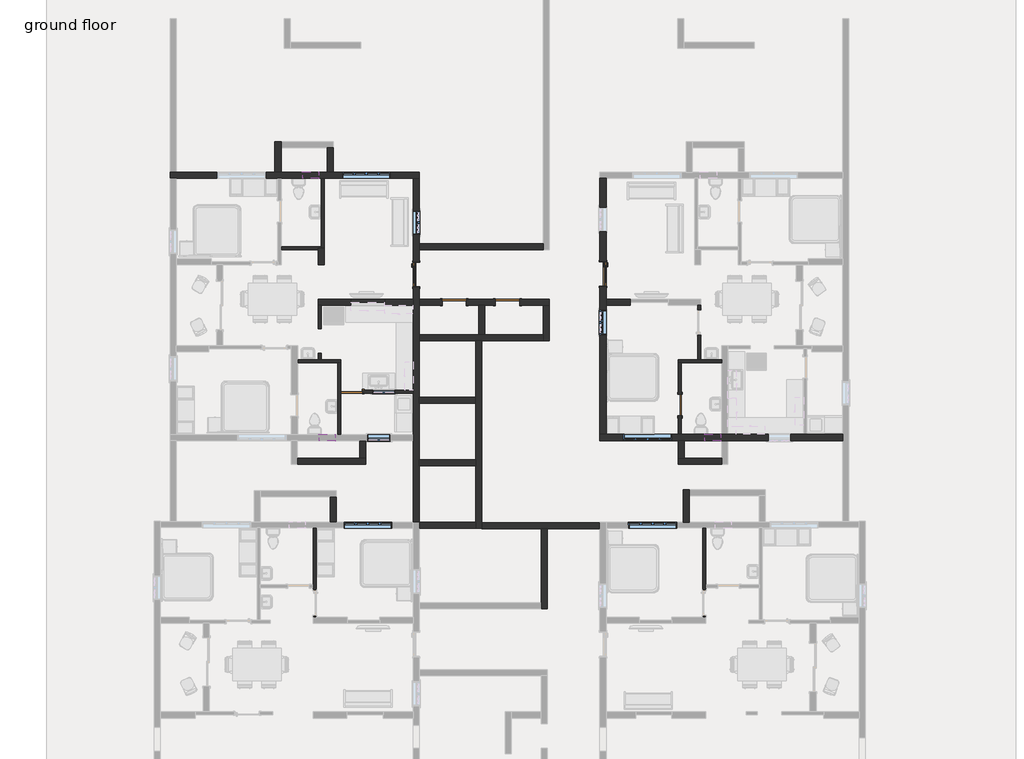
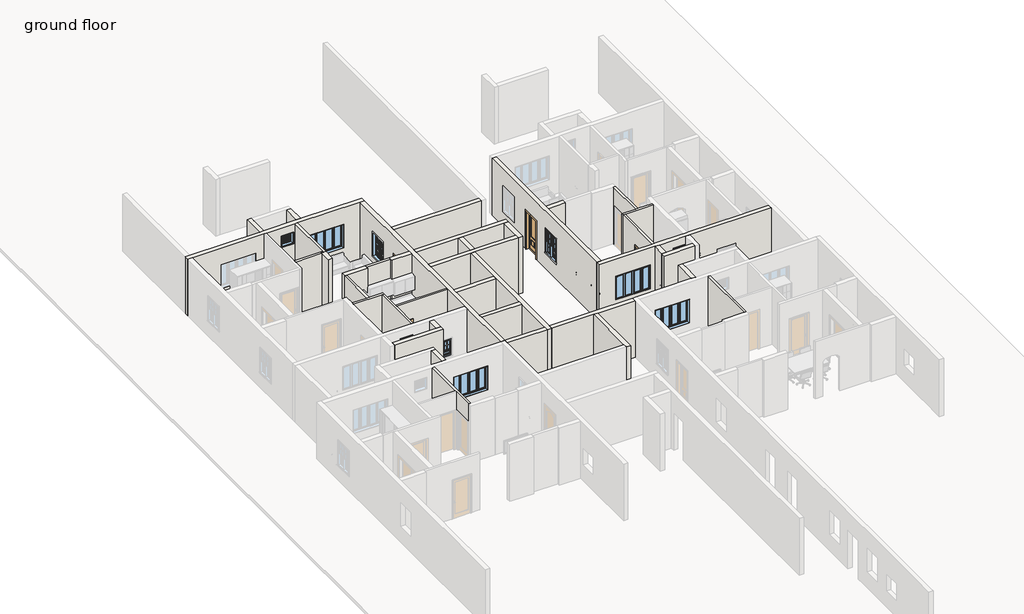
# One storey, part 5 of 16: 39 walls, 11 windows, 6 doors.
"""IFC4 building model written with IfcOpenShell, lengths in millimetres."""

from ifc_helpers import new_model, si_unit, point, frame, origin, place, context, project, spatial, polyline, ellipse_curve, trimmed, outline, extrude, faceted_brep, transform, mapped, element, save
from ifc_brep_helpers import plane_surface, extruded_surface, advanced_brep
from components import door_fe8ae985, door_f079f64e, door_38851409, door_d141acb4, door_0ca8825f, window_ced37e8f, window_622386c7, window_5487fb6d, window_f2d8fef0, window_45970670

model = new_model("IFC4")

# Units and contexts
model_context = context("Model", 3, world=origin())
ifc_project = project(units=[si_unit("LENGTHUNIT", "METRE", prefix="MILLI")], contexts=[model_context])

# Site, building, storey
site = spatial("IfcSite", under=ifc_project)
building = spatial("IfcBuilding", under=site)
storey = spatial("IfcBuildingStorey", under=building, Name="ground floor", Elevation=609.6)

# Doors
placement = place(None, origin())
door_shape = door_fe8ae985(model_context)
element("IfcDoor", 1, ObjectType="36\" x 84\"", at=placement, inside=storey, context=model_context, shape_type="MappedRepresentation", body=[
    mapped(door_shape, transform((59474.0062819, 11381.8650652, 609.6), x_axis=(0.0, 1.0, 0.0), y_axis=(-1.0, 0.0, 0.0), z_axis=(0.0, 0.0, 1.0))),
])
door_2_shape = door_f079f64e(model_context)
element("IfcDoor", 2, ObjectType="36\" x 84\"", at=placement, inside=storey, context=model_context, shape_type="MappedRepresentation", body=[
    mapped(door_2_shape, transform((52422.151243, 11359.5034272, 609.6), x_axis=(0.0, 1.0, 0.0), y_axis=(-1.0, 0.0, 0.0), z_axis=(0.0, 0.0, 1.0))),
])
door_3_shape = door_38851409(model_context)
element("IfcDoor", 3, ObjectType="Single-Flush : 32\" x 84\"", at=placement, inside=storey, context=model_context, shape_type="MappedRepresentation", body=[
    mapped(door_3_shape, transform((62372.7812819, 6428.8650652, 609.6), x_axis=(0.0, 1.0, 0.0), y_axis=(-1.0, 0.0, 0.0), z_axis=(0.0, 0.0, 1.0))),
])
door_4_shape = door_d141acb4(model_context)
element("IfcDoor", 4, ObjectType="Single-Flush : 32\" x 84\"", at=placement, inside=storey, context=model_context, shape_type="MappedRepresentation", body=[
    mapped(door_4_shape, transform((49980.576243, 6943.2150652, 609.6), x_axis=(-1.0, 0.0, 0.0), y_axis=(0.0, -1.0, 0.0), z_axis=(0.0, 0.0, 1.0))),
])
door_5_shape = door_0ca8825f(model_context)
element("IfcDoor", 5, ObjectType="Single-Flush : 36\" x 84\"", at=placement, inside=storey, context=model_context, shape_type="MappedRepresentation", body=[
    mapped(door_5_shape, transform((55864.0312819, 10315.0650652, 609.6), x_axis=(1.0, 0.0, 0.0), y_axis=(0.0, 1.0, 0.0), z_axis=(0.0, 0.0, 1.0))),
])
element("IfcDoor", 6, ObjectType="Single-Flush : 36\" x 84\"", at=placement, inside=storey, context=model_context, shape_type="MappedRepresentation", body=[
    mapped(door_5_shape, transform((53857.4312819, 10315.0650652, 609.6), x_axis=(1.0, 0.0, 0.0), y_axis=(0.0, 1.0, 0.0), z_axis=(0.0, 0.0, 1.0))),
])

# Walls
element("IfcWall", 7, ObjectType="Generic - 4.5\"", at=placement, inside=storey, context=model_context, shape_type="Brep", body=[
    faceted_brep([(48843.926243, 14998.0718163, 609.6), (48843.926243, 12410.5650652, 609.6), (48843.926243, 12353.4150652, 609.6), (48843.926243, 12353.4150652, 3810.0), (48843.926243, 12410.5650652, 3810.0), (48843.926243, 14998.0718163, 3810.0), (48958.226243, 14998.0718163, 609.6), (48958.226243, 14998.0718163, 3810.0), (48958.226243, 12353.4150652, 3810.0), (48958.226243, 12353.4150652, 609.6)], [[[0, 1, 2, 3, 4, 5]], [[6, 7, 8, 9]], [[2, 1, 0, 6, 9]], [[3, 2, 9, 8]], [[5, 4, 3, 8, 7]], [[0, 5, 7, 6]]]),
])
element("IfcWall", 8, ObjectType="Generic - 4.5\"", at=placement, inside=storey, context=model_context, shape_type="SweptSolid", body=[
    extrude(outline(polyline([(48729.626243, 12296.2650652), (47319.926243, 12296.2650652), (47319.926243, 12410.5650652), (48843.926243, 12410.5650652), (48843.926243, 12353.4150652), (48729.626243, 12353.4150652), (48729.626243, 12296.2650652)])), frame((0.0, 0.0, 609.6), z_axis=(0.0, 0.0, 1.0), x_axis=(1.0, 0.0, 0.0)), (0.0, 0.0, 1.0), 3200.4),
])
element("IfcWall", 9, ObjectType="Generic - 4.5\"", at=placement, inside=storey, context=model_context, shape_type="SweptSolid", body=[
    extrude(outline(polyline([(51230.5865418, 10315.0650652), (49954.5136957, 10315.0650652), (49954.5136957, 10429.3650652), (51230.5865418, 10429.3650652), (51230.5865418, 10315.0650652)])), frame((0.0, 0.0, 609.6), z_axis=(0.0, 0.0, 1.0), x_axis=(1.0, 0.0, 0.0)), (0.0, 0.0, 1.0), 3200.4),
])
element("IfcWall", 10, ObjectType="Generic - 4.5\"", at=placement, inside=storey, context=model_context, shape_type="AdvancedBrep", body=[
    advanced_brep(
    [(48729.626243, 10200.7650652, 609.6), (48729.626243, 9305.4150652, 609.6), (48729.626243, 9305.4150652, 2540.0), (48729.626243, 8391.0150652, 2540.0), (48729.626243, 8391.0150652, 609.6), (48729.626243, 8143.3650652, 609.6), (48729.626243, 8143.3650652, 3810.0), (48729.626243, 10200.7650652, 3810.0), (48843.926243, 9305.4150652, 2540.0), (48843.926243, 9305.4150652, 609.6), (48843.926243, 10200.7650652, 609.6), (48843.926243, 10200.7650652, 3810.0), (48843.926243, 8143.3650652, 3810.0), (48843.926243, 8143.3650652, 609.6), (48843.926243, 8391.0150652, 609.6), (48843.926243, 8391.0150652, 2540.0)],
    [
        (0, 1),
        (1, 2),
        (2, 3, ellipse_curve(frame((48729.626243, 8848.2150652, 2540.0), z_axis=(1.0, 0.0, 0.0), x_axis=(0.0, 1.0, 0.0)), 457.2, 203.2)),
        (3, 4),
        (4, 5),
        (5, 6),
        (6, 7),
        (7, 0),
        (8, 9),
        (9, 10),
        (10, 11),
        (11, 12),
        (12, 13),
        (13, 14),
        (14, 15),
        (15, 8, ellipse_curve(frame((48843.926243, 8848.2150652, 2540.0), z_axis=(-1.0, 0.0, 0.0), x_axis=(0.0, 1.0, 0.0)), 457.2, 203.2)),
        (13, 5),
        (4, 14),
        (9, 1),
        (0, 10),
        (6, 12),
        (11, 7),
        (2, 8),
        (15, 3),
    ],
    [
        plane_surface(frame((48729.626243, 10200.7650652, 609.6), z_axis=(-1.0, 0.0, 0.0), x_axis=(0.0, -1.0, 0.0))),
        plane_surface(frame((48843.926243, 10200.7650652, 609.6), z_axis=(1.0, 0.0, 0.0), x_axis=(0.0, 1.0, 0.0))),
        plane_surface(frame((48729.626243, 10315.0650652, 609.6), z_axis=(0.0, 0.0, -1.0), x_axis=(1.0, 0.0, 0.0))),
        plane_surface(frame((48729.626243, 8086.2150652, 3810.0), z_axis=(0.0, 0.0, 1.0), x_axis=(1.0, 0.0, 0.0))),
        plane_surface(frame((48729.626243, 10200.7650652, 609.6), z_axis=(0.0, 1.0, 0.0), x_axis=(1.0, 0.0, 0.0))),
        plane_surface(frame((47942.226243, 8143.3650652, 609.6), z_axis=(0.0, -1.0, 0.0), x_axis=(-1.0, 0.0, 0.0))),
        extruded_surface(trimmed(ellipse_curve(frame((48958.226243, 8848.2150652, 2540.0), z_axis=(1.0, 0.0, 0.0), x_axis=(0.0, 1.0, 0.0)), 457.2, 203.2), [point((48958.226243, 9305.4150652, 2540.0))], [point((48958.226243, 8391.0150652, 2540.0))], True, "CARTESIAN"), (-114.29999999999563, 0.0, 0.0), 114.29999999999563),
        plane_surface(frame((48729.626243, 8391.0150652, 2540.0), z_axis=(0.0, 1.0, 0.0), x_axis=(1.0, 0.0, 0.0))),
        plane_surface(frame((48729.626243, 9305.4150652, 609.6), z_axis=(0.0, -1.0, 0.0), x_axis=(1.0, 0.0, 0.0))),
    ],
    [
        (0, [[1, 2, 3, 4, 5, 6, 7, 8]]),
        (1, [[9, 10, 11, 12, 13, 14, 15, 16]]),
        (2, [[-14, 17, -5, 18]]),
        (2, [[-10, 19, -1, 20]]),
        (3, [[-7, 21, -12, 22]]),
        (4, [[-8, -22, -11, -20]]),
        (5, [[-6, -17, -13, -21]]),
        (6, [[-3, 23, -16, 24]]),
        (7, [[-4, -24, -15, -18]]),
        (8, [[-2, -19, -9, -23]]),
    ],
),
])
element("IfcWall", 11, ObjectType="Generic - 4.5\"", at=placement, inside=storey, context=model_context, shape_type="Brep", body=[
    faceted_brep([(47942.226243, 8029.0650652, 609.6), (49466.226243, 8029.0650652, 609.6), (49580.526243, 8029.0650652, 609.6), (49580.526243, 8029.0650652, 3810.0), (49466.226243, 8029.0650652, 3810.0), (47942.226243, 8029.0650652, 3810.0), (47942.226243, 8143.3650652, 609.6), (47942.226243, 8143.3650652, 3810.0), (48729.626243, 8143.3650652, 3810.0), (48843.926243, 8143.3650652, 3810.0), (49580.526243, 8143.3650652, 3810.0), (49580.526243, 8143.3650652, 609.6), (48843.926243, 8143.3650652, 609.6), (48729.626243, 8143.3650652, 609.6)], [[[0, 1, 2, 3, 4, 5]], [[6, 7, 8, 9, 10, 11, 12, 13]], [[2, 1, 0, 6, 13, 12, 11]], [[5, 4, 3, 10, 9, 8, 7]], [[0, 5, 7, 6]], [[3, 2, 11, 10]]]),
])
element("IfcWall", 12, ObjectType="Generic - 4.5\"", at=placement, inside=storey, context=model_context, shape_type="Brep", body=[
    faceted_brep([(49466.226243, 8029.0650652, 609.6), (49466.226243, 5320.6718163, 609.6), (49466.226243, 5320.6718163, 3810.0), (49466.226243, 8029.0650652, 3810.0), (49580.526243, 8029.0650652, 3810.0), (49580.526243, 7000.3650652, 3810.0), (49580.526243, 6886.0650652, 3810.0), (49580.526243, 5320.6718163, 3810.0), (49580.526243, 5320.6718163, 609.6), (49580.526243, 6886.0650652, 609.6), (49580.526243, 6886.0650652, 2743.2), (49580.526243, 7000.3650652, 2743.2), (49580.526243, 7000.3650652, 609.6), (49580.526243, 8029.0650652, 609.6), (49574.176243, 7000.3650652, 609.6), (49574.176243, 6886.0650652, 609.6), (49574.176243, 7000.3650652, 2743.2), (49574.176243, 6886.0650652, 2743.2)], [[[0, 1, 2, 3]], [[4, 5, 6, 7, 8, 9, 10, 11, 12, 13]], [[1, 0, 13, 12, 14, 15, 9, 8]], [[3, 2, 7, 6, 5, 4]], [[0, 3, 4, 13]], [[2, 1, 8, 7]], [[16, 14, 12, 11]], [[15, 17, 10, 9]], [[14, 16, 17, 15]], [[17, 16, 11, 10]]]),
])
element("IfcWall", 13, ObjectType="Generic - 4.5\"", at=placement, inside=storey, context=model_context, shape_type="SweptSolid", body=[
    extrude(outline(polyline([(3810.0, 52311.026243), (3810.0, 49580.526243), (2743.2, 49580.526243), (2743.2, 50386.976243), (609.6, 50386.976243), (609.6, 52311.026243), (3810.0, 52311.026243)]), holes=[polyline([(2438.4, 50771.151243), (2438.4, 51634.751243), (1524.0, 51634.751243), (1524.0, 50771.151243), (2438.4, 50771.151243)])]), frame((0.0, 6886.0650652, 0.0), z_axis=(0.0, 1.0, 0.0), x_axis=(0.0, 0.0, 1.0)), (0.0, 0.0, 1.0), 114.3),
])
element("IfcWall", 14, ObjectType="Generic - 4.5\"", at=placement, inside=storey, context=model_context, shape_type="Brep", body=[
    faceted_brep([(63953.9312819, 8143.3650652, 609.6), (63166.5312819, 8143.3650652, 609.6), (63052.2312819, 8143.3650652, 609.6), (62315.6312819, 8143.3650652, 609.6), (62315.6312819, 8143.3650652, 3810.0), (63052.2312819, 8143.3650652, 3810.0), (63166.5312819, 8143.3650652, 3810.0), (63953.9312819, 8143.3650652, 3810.0), (63953.9312819, 8029.0650652, 609.6), (63953.9312819, 8029.0650652, 3810.0), (62429.9312819, 8029.0650652, 3810.0), (62315.6312819, 8029.0650652, 3810.0), (62315.6312819, 8029.0650652, 609.6), (62429.9312819, 8029.0650652, 609.6)], [[[0, 1, 2, 3, 4, 5, 6, 7]], [[8, 9, 10, 11, 12, 13]], [[3, 2, 1, 0, 8, 13, 12]], [[7, 6, 5, 4, 11, 10, 9]], [[0, 7, 9, 8]], [[4, 3, 12, 11]]]),
])
element("IfcWall", 15, ObjectType="Generic - 4.5\"", at=placement, inside=storey, context=model_context, shape_type="SweptSolid", body=[
    extrude(outline(polyline([(8029.0650652, 609.6), (6835.2650652, 609.6), (6835.2650652, 2743.2), (6022.4650652, 2743.2), (6022.4650652, 609.6), (5323.9650652, 609.6), (5323.9650652, 3810.0), (8029.0650652, 3810.0), (8029.0650652, 609.6)])), frame((62315.6312819, 0.0, 0.0), z_axis=(1.0, 0.0, 0.0), x_axis=(0.0, 1.0, 0.0)), (0.0, 0.0, 1.0), 114.3),
])
element("IfcWall", 16, ObjectType="Generic - 4.5\"", at=placement, inside=storey, context=model_context, shape_type="SweptSolid", body=[
    extrude(outline(polyline([(8143.3650652, 3810.0), (10200.7650652, 3810.0), (10200.7650652, 609.6), (10035.6650652, 609.6), (10035.6650652, 2768.6), (9070.4650652, 2768.6), (9070.4650652, 609.6), (8143.3650652, 609.6), (8143.3650652, 3810.0)])), frame((63052.2312819, 0.0, 0.0), z_axis=(1.0, 0.0, 0.0), x_axis=(0.0, 1.0, 0.0)), (0.0, 0.0, 1.0), 114.3),
])
element("IfcWall", 17, ObjectType="Generic - 4.5\"", at=placement, inside=storey, context=model_context, shape_type="Brep", body=[
    faceted_brep([(48539.126243, -1566.0113664, 3810.0), (48539.126243, -461.1113664, 3810.0), (48539.126243, -346.8113664, 3810.0), (48539.126243, 1794.3724636, 3810.0), (48539.126243, 1794.3724636, 609.6), (48539.126243, -346.8113664, 609.6), (48539.126243, -461.1113664, 609.6), (48539.126243, -559.5363664, 609.6), (48539.126243, -559.5363664, 2768.6), (48539.126243, -1524.7363664, 2768.6), (48539.126243, -1524.7363664, 609.6), (48539.126243, -1566.0113664, 609.6), (48653.426243, 1793.9176995, 3810.0), (48653.426243, -1566.0113664, 3810.0), (48653.426243, -1566.0113664, 609.6), (48653.426243, -1524.7363664, 609.6), (48653.426243, -1524.7363664, 2768.6), (48653.426243, -559.5363664, 2768.6), (48653.426243, -559.5363664, 609.6), (48653.426243, 1793.9176995, 609.6)], [[[0, 1, 2, 3, 4, 5, 6, 7, 8, 9, 10, 11]], [[12, 13, 14, 15, 16, 17, 18, 19]], [[4, 19, 18, 7, 6, 5]], [[14, 11, 10, 15]], [[3, 2, 1, 0, 13, 12]], [[0, 11, 14, 13]], [[4, 3, 12, 19]], [[9, 16, 15, 10]], [[16, 9, 8, 17]], [[17, 8, 7, 18]]]),
])
element("IfcWall", 18, ObjectType="Generic - 4.5\"", at=placement, inside=storey, context=model_context, shape_type="Brep", body=[
    faceted_brep([(63242.7312819, -1566.0113664, 3810.0), (63242.7312819, 1793.9176995, 3810.0), (63242.7312819, 1793.9176995, 609.6), (63242.7312819, -559.5363664, 609.6), (63242.7312819, -559.5363664, 2768.6), (63242.7312819, -1524.7363664, 2768.6), (63242.7312819, -1524.7363664, 609.6), (63242.7312819, -1566.0113664, 609.6), (63357.0312819, 1794.3724636, 3810.0), (63357.0312819, -346.8113664, 3810.0), (63357.0312819, -461.1113664, 3810.0), (63357.0312819, -1566.0113664, 3810.0), (63357.0312819, -1566.0113664, 609.6), (63357.0312819, -1524.7363664, 609.6), (63357.0312819, -1524.7363664, 2768.6), (63357.0312819, -559.5363664, 2768.6), (63357.0312819, -559.5363664, 609.6), (63357.0312819, -461.1113664, 609.6), (63357.0312819, -346.8113664, 609.6), (63357.0312819, 1794.3724636, 609.6)], [[[0, 1, 2, 3, 4, 5, 6, 7]], [[8, 9, 10, 11, 12, 13, 14, 15, 16, 17, 18, 19]], [[2, 19, 18, 17, 16, 3]], [[12, 7, 6, 13]], [[1, 0, 11, 10, 9, 8]], [[0, 7, 12, 11]], [[2, 1, 8, 19]], [[5, 14, 13, 6]], [[14, 5, 4, 15]], [[15, 4, 3, 16]]]),
])
element("IfcWall", 19, ObjectType="Generic - 9\"", at=placement, inside=storey, context=model_context, shape_type="Brep", body=[
    faceted_brep([(43141.626243, 14998.0718163, 609.6), (43370.226243, 14998.0718163, 609.6), (47205.626243, 14998.0718163, 609.6), (47319.926243, 14998.0718163, 609.6), (48843.926243, 14998.0718163, 609.6), (48958.226243, 14998.0718163, 609.6), (52311.026243, 14998.0718163, 609.6), (52539.626243, 14998.0718163, 609.6), (52539.626243, 14998.0718163, 3810.0), (52311.026243, 14998.0718163, 3810.0), (48958.226243, 14998.0718163, 3810.0), (48843.926243, 14998.0718163, 3810.0), (47319.926243, 14998.0718163, 3810.0), (47205.626243, 14998.0718163, 3810.0), (43370.226243, 14998.0718163, 3810.0), (43141.626243, 14998.0718163, 3810.0), (46748.426243, 14998.0718163, 2870.2), (46748.426243, 14998.0718163, 1524.0), (44919.626243, 14998.0718163, 1524.0), (44919.626243, 14998.0718163, 2870.2), (51457.2877548, 14998.0718163, 2870.2), (51457.2877548, 14998.0718163, 1524.0), (49628.4877548, 14998.0718163, 1524.0), (49628.4877548, 14998.0718163, 2870.2), (48139.076243, 14998.0718163, 3352.8), (48748.676243, 14998.0718163, 3352.8), (48748.676243, 14998.0718163, 2743.2), (48139.076243, 14998.0718163, 2743.2), (43141.626243, 15226.6718163, 609.6), (43141.626243, 15226.6718163, 3810.0), (43370.226243, 15226.6718163, 3810.0), (47091.326243, 15226.6718163, 3810.0), (47319.926243, 15226.6718163, 3810.0), (49056.9877548, 15226.6718163, 3810.0), (49285.5877548, 15226.6718163, 3810.0), (52539.626243, 15226.6718163, 3810.0), (52539.626243, 15226.6718163, 609.6), (49285.5877548, 15226.6718163, 609.6), (49056.9877548, 15226.6718163, 609.6), (47319.926243, 15226.6718163, 609.6), (47091.326243, 15226.6718163, 609.6), (43370.226243, 15226.6718163, 609.6), (46748.426243, 15226.6718163, 2870.2), (44919.626243, 15226.6718163, 2870.2), (44919.626243, 15226.6718163, 1524.0), (46748.426243, 15226.6718163, 1524.0), (51457.2877548, 15226.6718163, 2870.2), (49628.4877548, 15226.6718163, 2870.2), (49628.4877548, 15226.6718163, 1524.0), (51457.2877548, 15226.6718163, 1524.0), (48139.076243, 15226.6718163, 3352.8), (48139.076243, 15226.6718163, 2743.2), (48748.676243, 15226.6718163, 2743.2), (48748.676243, 15226.6718163, 3352.8)], [[[0, 1, 2, 3, 4, 5, 6, 7, 8, 9, 10, 11, 12, 13, 14, 15], [16, 17, 18, 19], [20, 21, 22, 23], [24, 25, 26, 27]], [[28, 29, 30, 31, 32, 33, 34, 35, 36, 37, 38, 39, 40, 41], [42, 43, 44, 45], [46, 47, 48, 49], [50, 51, 52, 53]], [[7, 6, 5, 4, 3, 2, 1, 0, 28, 41, 40, 39, 38, 37, 36]], [[15, 14, 13, 12, 11, 10, 9, 8, 35, 34, 33, 32, 31, 30, 29]], [[8, 7, 36, 35]], [[0, 15, 29, 28]], [[17, 16, 42, 45]], [[18, 17, 45, 44]], [[19, 18, 44, 43]], [[16, 19, 43, 42]], [[21, 20, 46, 49]], [[22, 21, 49, 48]], [[23, 22, 48, 47]], [[20, 23, 47, 46]], [[51, 50, 24, 27]], [[52, 51, 27, 26]], [[53, 52, 26, 25]], [[50, 53, 25, 24]]]),
])
element("IfcWall", 20, ObjectType="Generic - 9\"", at=placement, inside=storey, context=model_context, shape_type="Brep", body=[
    faceted_brep([(52311.026243, 2007.967056, 3810.0), (52311.026243, 5092.0718163, 3810.0), (52311.026243, 5320.6718163, 3810.0), (52311.026243, 6886.0650652, 3810.0), (52311.026243, 7000.3650652, 3810.0), (52311.026243, 10200.7650652, 3810.0), (52311.026243, 10429.3650652, 3810.0), (52311.026243, 14998.0718163, 3810.0), (52311.026243, 14998.0718163, 609.6), (52311.026243, 11842.1034272, 609.6), (52311.026243, 11842.1034272, 2768.6), (52311.026243, 10876.9034272, 2768.6), (52311.026243, 10876.9034272, 609.6), (52311.026243, 10429.3650652, 609.6), (52311.026243, 10200.7650652, 609.6), (52311.026243, 7000.3650652, 609.6), (52311.026243, 6886.0650652, 609.6), (52311.026243, 5320.6718163, 609.6), (52311.026243, 5092.0718163, 609.6), (52311.026243, 2007.967056, 609.6), (52311.026243, 13775.5417893, 2844.8), (52311.026243, 12861.1417893, 2844.8), (52311.026243, 12861.1417893, 1524.0), (52311.026243, 13775.5417893, 1524.0), (52539.626243, 14998.0718163, 3810.0), (52539.626243, 12518.2417893, 3810.0), (52539.626243, 12289.6417893, 3810.0), (52539.626243, 10429.3650652, 3810.0), (52539.626243, 10200.7650652, 3810.0), (52539.626243, 9093.6575277, 3810.0), (52539.626243, 8865.0575277, 3810.0), (52539.626243, 6731.4575277, 3810.0), (52539.626243, 6502.8575277, 3810.0), (52539.626243, 4369.2575277, 3810.0), (52539.626243, 4140.6575277, 3810.0), (52539.626243, 2007.0575277, 3810.0), (52539.626243, 2007.0575277, 609.6), (52539.626243, 4140.6575277, 609.6), (52539.626243, 4369.2575277, 609.6), (52539.626243, 6502.8575277, 609.6), (52539.626243, 6731.4575277, 609.6), (52539.626243, 8865.0575277, 609.6), (52539.626243, 9093.6575277, 609.6), (52539.626243, 10200.7650652, 609.6), (52539.626243, 10429.3650652, 609.6), (52539.626243, 10876.9034272, 609.6), (52539.626243, 10876.9034272, 2768.6), (52539.626243, 11842.1034272, 2768.6), (52539.626243, 11842.1034272, 609.6), (52539.626243, 12289.6417893, 609.6), (52539.626243, 12518.2417893, 609.6), (52539.626243, 14998.0718163, 609.6), (52539.626243, 13775.5417893, 2844.8), (52539.626243, 13775.5417893, 1524.0), (52539.626243, 12861.1417893, 1524.0), (52539.626243, 12861.1417893, 2844.8)], [[[0, 1, 2, 3, 4, 5, 6, 7, 8, 9, 10, 11, 12, 13, 14, 15, 16, 17, 18, 19], [20, 21, 22, 23]], [[24, 25, 26, 27, 28, 29, 30, 31, 32, 33, 34, 35, 36, 37, 38, 39, 40, 41, 42, 43, 44, 45, 46, 47, 48, 49, 50, 51], [52, 53, 54, 55]], [[8, 51, 50, 49, 48, 9]], [[36, 19, 18, 17, 16, 15, 14, 13, 12, 45, 44, 43, 42, 41, 40, 39, 38, 37]], [[7, 6, 5, 4, 3, 2, 1, 0, 35, 34, 33, 32, 31, 30, 29, 28, 27, 26, 25, 24]], [[8, 7, 24, 51]], [[0, 19, 36, 35]], [[47, 10, 9, 48]], [[10, 47, 46, 11]], [[11, 46, 45, 12]], [[53, 52, 20, 23]], [[54, 53, 23, 22]], [[55, 54, 22, 21]], [[52, 55, 21, 20]]]),
])
element("IfcWall", 21, ObjectType="Generic - 9\"", at=placement, inside=storey, context=model_context, shape_type="Brep", body=[
    faceted_brep([(48729.626243, 10200.7650652, 609.6), (48843.926243, 10200.7650652, 609.6), (49954.5136957, 10200.7650652, 609.6), (49954.5136957, 10200.7650652, 3810.0), (48843.926243, 10200.7650652, 3810.0), (48729.626243, 10200.7650652, 3810.0), (48729.626243, 10429.3650652, 609.6), (48729.626243, 10429.3650652, 3810.0), (49954.5136957, 10429.3650652, 3810.0), (49954.5136957, 10429.3650652, 609.6), (49954.5136957, 10315.0650652, 609.6), (49954.5136957, 10315.0650652, 3810.0)], [[[0, 1, 2, 3, 4, 5]], [[6, 7, 8, 9]], [[2, 1, 0, 6, 9, 10]], [[3, 2, 10, 9, 8, 11]], [[5, 4, 3, 11, 8, 7]], [[0, 5, 7, 6]]]),
])
element("IfcWall", 22, ObjectType="Generic - 9\"", at=placement, inside=storey, context=model_context, shape_type="Brep", body=[
    faceted_brep([(51230.5865418, 10200.7650652, 609.6), (52311.026243, 10200.7650652, 609.6), (52311.026243, 10200.7650652, 3810.0), (51230.5865418, 10200.7650652, 3810.0), (51230.5865418, 10429.3650652, 609.6), (51230.5865418, 10429.3650652, 3810.0), (52311.026243, 10429.3650652, 3810.0), (52311.026243, 10429.3650652, 609.6), (51230.5865418, 10315.0650652, 609.6), (51230.5865418, 10315.0650652, 3810.0)], [[[0, 1, 2, 3]], [[4, 5, 6, 7]], [[1, 0, 8, 4, 7]], [[3, 2, 6, 5, 9]], [[0, 3, 9, 5, 4, 8]], [[2, 1, 7, 6]]]),
])
element("IfcWall", 23, ObjectType="Generic - 9\"", at=placement, inside=storey, context=model_context, shape_type="Brep", body=[
    faceted_brep([(48958.226243, 11724.7650652, 609.6), (48958.226243, 12353.4150652, 609.6), (48958.226243, 12353.4150652, 3810.0), (48958.226243, 11724.7650652, 3810.0), (48729.626243, 11724.7650652, 609.6), (48729.626243, 11724.7650652, 3810.0), (48729.626243, 12296.2650652, 3810.0), (48729.626243, 12353.4150652, 3810.0), (48729.626243, 12353.4150652, 609.6), (48729.626243, 12296.2650652, 609.6), (48843.926243, 12353.4150652, 609.6), (48843.926243, 12353.4150652, 3810.0)], [[[0, 1, 2, 3]], [[4, 5, 6, 7, 8, 9]], [[1, 0, 4, 9, 8, 10]], [[2, 1, 10, 8, 7, 11]], [[3, 2, 11, 7, 6, 5]], [[0, 3, 5, 4]]]),
])
element("IfcWall", 24, ObjectType="Generic - 9\"", at=placement, inside=storey, context=model_context, shape_type="Brep", body=[
    faceted_brep([(47319.926243, 15226.6718163, 609.6), (47319.926243, 16147.8755101, 609.6), (47319.926243, 16376.4755101, 609.6), (47319.926243, 16376.4755101, 3810.0), (47319.926243, 16147.8755101, 3810.0), (47319.926243, 15226.6718163, 3810.0), (47091.326243, 15226.6718163, 609.6), (47091.326243, 15226.6718163, 3810.0), (47091.326243, 16376.4755101, 3810.0), (47091.326243, 16376.4755101, 609.6)], [[[0, 1, 2, 3, 4, 5]], [[6, 7, 8, 9]], [[2, 1, 0, 6, 9]], [[5, 4, 3, 8, 7]], [[0, 5, 7, 6]], [[3, 2, 9, 8]]]),
])
element("IfcWall", 25, ObjectType="Generic - 9\"", at=placement, inside=storey, context=model_context, shape_type="SweptSolid", body=[
    extrude(outline(polyline([(49056.9877548, 15226.6718163), (49056.9877548, 16147.8755101), (49285.5877548, 16147.8755101), (49285.5877548, 15226.6718163), (49056.9877548, 15226.6718163)])), frame((0.0, 0.0, 609.6), z_axis=(0.0, 0.0, 1.0), x_axis=(1.0, 0.0, 0.0)), (0.0, 0.0, 1.0), 3200.4),
])
element("IfcWall", 26, ObjectType="Generic - 9\"", at=placement, inside=storey, context=model_context, shape_type="Brep", body=[
    faceted_brep([(47929.526243, 4203.0718163, 609.6), (50519.795833, 4203.0718163, 609.6), (50519.795833, 4203.0718163, 3810.0), (47929.526243, 4203.0718163, 3810.0), (47929.526243, 4431.6718163, 609.6), (47929.526243, 4431.6718163, 3810.0), (50291.195833, 4431.6718163, 3810.0), (50519.795833, 4431.6718163, 3810.0), (50519.795833, 4431.6718163, 609.6), (50291.195833, 4431.6718163, 609.6)], [[[0, 1, 2, 3]], [[4, 5, 6, 7, 8, 9]], [[1, 0, 4, 9, 8]], [[3, 2, 7, 6, 5]], [[0, 3, 5, 4]], [[2, 1, 8, 7]]]),
])
element("IfcWall", 27, ObjectType="Generic - 9\"", at=placement, inside=storey, context=model_context, shape_type="SweptSolid", body=[
    extrude(outline(polyline([(50519.795833, 5092.0718163), (50519.795833, 4431.6718163), (50291.195833, 4431.6718163), (50291.195833, 5092.0718163), (50519.795833, 5092.0718163)])), frame((0.0, 0.0, 609.6), z_axis=(0.0, 0.0, 1.0), x_axis=(1.0, 0.0, 0.0)), (0.0, 0.0, 1.0), 3200.4),
])
element("IfcWall", 28, ObjectType="Generic - 9\"", at=placement, inside=storey, context=model_context, shape_type="Brep", body=[
    faceted_brep([(68525.9312819, 5323.9650652, 609.6), (67154.3312819, 5323.9650652, 609.6), (67040.0312819, 5323.9650652, 609.6), (64182.5312819, 5323.9650652, 609.6), (63953.9312819, 5323.9650652, 609.6), (62429.9312819, 5323.9650652, 609.6), (62315.6312819, 5323.9650652, 609.6), (59585.1312819, 5323.9650652, 609.6), (59356.5312819, 5323.9650652, 609.6), (59356.5312819, 5323.9650652, 3810.0), (59585.1312819, 5323.9650652, 3810.0), (62315.6312819, 5323.9650652, 3810.0), (62429.9312819, 5323.9650652, 3810.0), (63953.9312819, 5323.9650652, 3810.0), (64182.5312819, 5323.9650652, 3810.0), (67040.0312819, 5323.9650652, 3810.0), (67154.3312819, 5323.9650652, 3810.0), (68525.9312819, 5323.9650652, 3810.0), (60239.1812819, 5323.9650652, 2870.2), (60239.1812819, 5323.9650652, 1524.0), (62067.9812819, 5323.9650652, 1524.0), (62067.9812819, 5323.9650652, 2870.2), (65700.1812819, 5323.9650652, 2438.4), (65700.1812819, 5323.9650652, 1524.0), (66563.7812819, 5323.9650652, 1524.0), (66563.7812819, 5323.9650652, 2438.4), (63915.8312819, 5323.9650652, 3352.8), (63306.2312819, 5323.9650652, 3352.8), (63306.2312819, 5323.9650652, 2743.2), (63915.8312819, 5323.9650652, 2743.2), (68525.9312819, 5095.3650652, 609.6), (68525.9312819, 5095.3650652, 3810.0), (64182.5312819, 5095.3650652, 3810.0), (63953.9312819, 5095.3650652, 3810.0), (62544.2312819, 5095.3650652, 3810.0), (62315.6312819, 5095.3650652, 3810.0), (59356.5312819, 5095.3650652, 3810.0), (59356.5312819, 5095.3650652, 609.6), (62315.6312819, 5095.3650652, 609.6), (62544.2312819, 5095.3650652, 609.6), (63953.9312819, 5095.3650652, 609.6), (64182.5312819, 5095.3650652, 609.6), (60239.1812819, 5095.3650652, 2870.2), (62067.9812819, 5095.3650652, 2870.2), (62067.9812819, 5095.3650652, 1524.0), (60239.1812819, 5095.3650652, 1524.0), (65700.1812819, 5095.3650652, 2438.4), (66563.7812819, 5095.3650652, 2438.4), (66563.7812819, 5095.3650652, 1524.0), (65700.1812819, 5095.3650652, 1524.0), (63915.8312819, 5095.3650652, 3352.8), (63915.8312819, 5095.3650652, 2743.2), (63306.2312819, 5095.3650652, 2743.2), (63306.2312819, 5095.3650652, 3352.8)], [[[0, 1, 2, 3, 4, 5, 6, 7, 8, 9, 10, 11, 12, 13, 14, 15, 16, 17], [18, 19, 20, 21], [22, 23, 24, 25], [26, 27, 28, 29]], [[30, 31, 32, 33, 34, 35, 36, 37, 38, 39, 40, 41], [42, 43, 44, 45], [46, 47, 48, 49], [50, 51, 52, 53]], [[8, 7, 6, 5, 4, 3, 2, 1, 0, 30, 41, 40, 39, 38, 37]], [[17, 16, 15, 14, 13, 12, 11, 10, 9, 36, 35, 34, 33, 32, 31]], [[0, 17, 31, 30]], [[9, 8, 37, 36]], [[19, 18, 42, 45]], [[20, 19, 45, 44]], [[21, 20, 44, 43]], [[18, 21, 43, 42]], [[23, 22, 46, 49]], [[24, 23, 49, 48]], [[25, 24, 48, 47]], [[22, 25, 47, 46]], [[51, 50, 26, 29]], [[52, 51, 29, 28]], [[53, 52, 28, 27]], [[50, 53, 27, 26]]]),
])
element("IfcWall", 29, ObjectType="Generic - 9\"", at=placement, inside=storey, context=model_context, shape_type="Brep", body=[
    faceted_brep([(59585.1312819, 15001.3650652, 3810.0), (59585.1312819, 10429.3650652, 3810.0), (59585.1312819, 10200.7650652, 3810.0), (59585.1312819, 5323.9650652, 3810.0), (59585.1312819, 5323.9650652, 609.6), (59585.1312819, 10200.7650652, 609.6), (59585.1312819, 10429.3650652, 609.6), (59585.1312819, 10899.2650652, 609.6), (59585.1312819, 10899.2650652, 2768.6), (59585.1312819, 11864.4650652, 2768.6), (59585.1312819, 11864.4650652, 609.6), (59585.1312819, 15001.3650652, 609.6), (59585.1312819, 12982.0650652, 2844.8), (59585.1312819, 13896.4650652, 2844.8), (59585.1312819, 13896.4650652, 1524.0), (59585.1312819, 12982.0650652, 1524.0), (59585.1312819, 9095.8650652, 2844.8), (59585.1312819, 10010.2650652, 2844.8), (59585.1312819, 10010.2650652, 1524.0), (59585.1312819, 9095.8650652, 1524.0), (59356.5312819, 5323.9650652, 3810.0), (59356.5312819, 15001.3650652, 3810.0), (59356.5312819, 15001.3650652, 609.6), (59356.5312819, 11864.4650652, 609.6), (59356.5312819, 11864.4650652, 2768.6), (59356.5312819, 10899.2650652, 2768.6), (59356.5312819, 10899.2650652, 609.6), (59356.5312819, 5323.9650652, 609.6), (59356.5312819, 12982.0650652, 2844.8), (59356.5312819, 12982.0650652, 1524.0), (59356.5312819, 13896.4650652, 1524.0), (59356.5312819, 13896.4650652, 2844.8), (59356.5312819, 9095.8650652, 2844.8), (59356.5312819, 9095.8650652, 1524.0), (59356.5312819, 10010.2650652, 1524.0), (59356.5312819, 10010.2650652, 2844.8)], [[[0, 1, 2, 3, 4, 5, 6, 7, 8, 9, 10, 11], [12, 13, 14, 15], [16, 17, 18, 19]], [[20, 21, 22, 23, 24, 25, 26, 27], [28, 29, 30, 31], [32, 33, 34, 35]], [[4, 27, 26, 7, 6, 5]], [[22, 11, 10, 23]], [[3, 2, 1, 0, 21, 20]], [[0, 11, 22, 21]], [[4, 3, 20, 27]], [[9, 24, 23, 10]], [[24, 9, 8, 25]], [[25, 8, 7, 26]], [[29, 28, 12, 15]], [[30, 29, 15, 14]], [[31, 30, 14, 13]], [[28, 31, 13, 12]], [[33, 32, 16, 19]], [[34, 33, 19, 18]], [[35, 34, 18, 17]], [[32, 35, 17, 16]]]),
])
element("IfcWall", 30, ObjectType="Generic - 9\"", at=placement, inside=storey, context=model_context, shape_type="Brep", body=[
    faceted_brep([(59585.1312819, 10200.7650652, 609.6), (60499.5312819, 10200.7650652, 609.6), (60499.5312819, 10200.7650652, 3810.0), (59585.1312819, 10200.7650652, 3810.0), (59585.1312819, 10429.3650652, 609.6), (59585.1312819, 10429.3650652, 3810.0), (60499.5312819, 10429.3650652, 3810.0), (60499.5312819, 10429.3650652, 609.6), (60499.5312819, 10315.0650652, 609.6), (60499.5312819, 10315.0650652, 3810.0)], [[[0, 1, 2, 3]], [[4, 5, 6, 7]], [[1, 0, 4, 7, 8]], [[2, 1, 8, 7, 6, 9]], [[3, 2, 9, 6, 5]], [[0, 3, 5, 4]]]),
])
element("IfcWall", 31, ObjectType="Generic - 9\"", at=placement, inside=storey, context=model_context, shape_type="Brep", body=[
    faceted_brep([(63953.9312819, 4428.1961185, 609.6), (62544.2312819, 4428.1961185, 609.6), (62315.6312819, 4428.1961185, 609.6), (62315.6312819, 4428.1961185, 3810.0), (62544.2312819, 4428.1961185, 3810.0), (63953.9312819, 4428.1961185, 3810.0), (63953.9312819, 4199.5961185, 609.6), (63953.9312819, 4199.5961185, 3810.0), (62315.6312819, 4199.5961185, 3810.0), (62315.6312819, 4199.5961185, 609.6)], [[[0, 1, 2, 3, 4, 5]], [[6, 7, 8, 9]], [[2, 1, 0, 6, 9]], [[5, 4, 3, 8, 7]], [[0, 5, 7, 6]], [[3, 2, 9, 8]]]),
])
element("IfcWall", 32, ObjectType="Generic - 9\"", at=placement, inside=storey, context=model_context, shape_type="SweptSolid", body=[
    extrude(outline(polyline([(62544.2312819, 5095.3650652), (62544.2312819, 4428.1961185), (62315.6312819, 4428.1961185), (62315.6312819, 5095.3650652), (62544.2312819, 5095.3650652)])), frame((0.0, 0.0, 609.6), z_axis=(0.0, 0.0, 1.0), x_axis=(1.0, 0.0, 0.0)), (0.0, 0.0, 1.0), 3200.4),
])
element("IfcWall", 33, ObjectType="Generic - 9\"", at=placement, inside=storey, context=model_context, shape_type="Brep", body=[
    faceted_brep([(62726.6739944, 2020.4662774, 609.6), (62726.6739944, 3010.1567491, 609.6), (62726.6739944, 3238.7567491, 609.6), (62726.6739944, 3238.7567491, 3810.0), (62726.6739944, 3010.1567491, 3810.0), (62726.6739944, 2020.4662774, 3810.0), (62498.0739944, 2019.5567491, 609.6), (62498.0739944, 2019.5567491, 3810.0), (62498.0739944, 3238.7567491, 3810.0), (62498.0739944, 3238.7567491, 609.6)], [[[0, 1, 2, 3, 4, 5]], [[6, 7, 8, 9]], [[2, 1, 0, 6, 9]], [[5, 4, 3, 8, 7]], [[0, 5, 7, 6]], [[3, 2, 9, 8]]]),
])
element("IfcWall", 34, ObjectType="Generic - 9\"", at=placement, inside=storey, context=model_context, shape_type="SweptSolid", body=[
    extrude(outline(polyline([(49173.3107305, 2020.4510502), (49173.3107305, 2979.67086), (49401.9107305, 2979.67086), (49401.9107305, 2019.5415219), (49173.3107305, 2020.4510502)])), frame((0.0, 0.0, 609.6), z_axis=(0.0, 0.0, 1.0), x_axis=(1.0, 0.0, 0.0)), (0.0, 0.0, 1.0), 3200.4),
])
element("IfcWall", 35, ObjectType="Generic - 9\"", at=placement, inside=storey, context=model_context, shape_type="SweptSolid", body=[
    extrude(outline(polyline([(52539.626243, 12518.2417893), (57222.9312819, 12518.2417893), (57222.9312819, 12289.6417893), (52539.626243, 12289.6417893), (52539.626243, 12518.2417893)])), frame((0.0, 0.0, 609.6), z_axis=(0.0, 0.0, 1.0), x_axis=(1.0, 0.0, 0.0)), (0.0, 0.0, 1.0), 3200.4),
])
element("IfcWall", 36, ObjectType="Generic - 9\"", at=placement, inside=storey, context=model_context, shape_type="Brep", body=[
    faceted_brep([(54314.6312819, 10200.7650652, 2743.2), (54314.6312819, 10200.7650652, 609.6), (54784.5312819, 10200.7650652, 609.6), (55013.1312819, 10200.7650652, 609.6), (55406.8312819, 10200.7650652, 609.6), (55406.8312819, 10200.7650652, 2743.2), (56321.2312819, 10200.7650652, 2743.2), (56321.2312819, 10200.7650652, 609.6), (57222.9312819, 10200.7650652, 609.6), (57451.5312819, 10200.7650652, 609.6), (57451.5312819, 10200.7650652, 3810.0), (57222.9312819, 10200.7650652, 3810.0), (55013.1312819, 10200.7650652, 3810.0), (54784.5312819, 10200.7650652, 3810.0), (52539.626243, 10200.7650652, 3810.0), (52539.626243, 10200.7650652, 609.6), (53400.2312819, 10200.7650652, 609.6), (53400.2312819, 10200.7650652, 2743.2), (55406.8312819, 10429.3650652, 609.6), (54314.6312819, 10429.3650652, 609.6), (54314.6312819, 10429.3650652, 2743.2), (53400.2312819, 10429.3650652, 2743.2), (53400.2312819, 10429.3650652, 609.6), (52539.626243, 10429.3650652, 609.6), (52539.626243, 10429.3650652, 3810.0), (57451.5312819, 10429.3650652, 3810.0), (57451.5312819, 10429.3650652, 609.6), (56321.2312819, 10429.3650652, 609.6), (56321.2312819, 10429.3650652, 2743.2), (55406.8312819, 10429.3650652, 2743.2)], [[[0, 1, 2, 3, 4, 5, 6, 7, 8, 9, 10, 11, 12, 13, 14, 15, 16, 17]], [[18, 19, 20, 21, 22, 23, 24, 25, 26, 27, 28, 29]], [[9, 8, 7, 27, 26]], [[16, 15, 23, 22]], [[4, 3, 2, 1, 19, 18]], [[14, 13, 12, 11, 10, 25, 24]], [[15, 14, 24, 23]], [[10, 9, 26, 25]], [[28, 27, 7, 6]], [[29, 28, 6, 5]], [[18, 29, 5, 4]], [[20, 19, 1, 0]], [[21, 20, 0, 17]], [[22, 21, 17, 16]]]),
])
element("IfcWall", 37, ObjectType="Generic - 9\"", at=placement, inside=storey, context=model_context, shape_type="Brep", body=[
    faceted_brep([(57222.9312819, 10200.7650652, 609.6), (57222.9312819, 9093.6575277, 609.6), (57222.9312819, 8865.0575277, 609.6), (57222.9312819, 8865.0575277, 3810.0), (57222.9312819, 9093.6575277, 3810.0), (57222.9312819, 10200.7650652, 3810.0), (57451.5312819, 10200.7650652, 609.6), (57451.5312819, 10200.7650652, 3810.0), (57451.5312819, 8865.0575277, 3810.0), (57451.5312819, 8865.0575277, 609.6)], [[[0, 1, 2, 3, 4, 5]], [[6, 7, 8, 9]], [[2, 1, 0, 6, 9]], [[5, 4, 3, 8, 7]], [[0, 5, 7, 6]], [[3, 2, 9, 8]]]),
])
element("IfcWall", 38, ObjectType="Generic - 9\"", at=placement, inside=storey, context=model_context, shape_type="Brep", body=[
    faceted_brep([(57222.9312819, 9093.6575277, 609.6), (55013.1312819, 9093.6575277, 609.6), (54784.5312819, 9093.6575277, 609.6), (52539.626243, 9093.6575277, 609.6), (52539.626243, 9093.6575277, 3810.0), (54784.5312819, 9093.6575277, 3810.0), (55013.1312819, 9093.6575277, 3810.0), (57222.9312819, 9093.6575277, 3810.0), (57222.9312819, 8865.0575277, 609.6), (57222.9312819, 8865.0575277, 3810.0), (54901.826243, 8865.0575277, 3810.0), (54673.226243, 8865.0575277, 3810.0), (52539.626243, 8865.0575277, 3810.0), (52539.626243, 8865.0575277, 609.6), (54673.226243, 8865.0575277, 609.6), (54901.826243, 8865.0575277, 609.6)], [[[0, 1, 2, 3, 4, 5, 6, 7]], [[8, 9, 10, 11, 12, 13, 14, 15]], [[3, 2, 1, 0, 8, 15, 14, 13]], [[7, 6, 5, 4, 12, 11, 10, 9]], [[0, 7, 9, 8]], [[4, 3, 13, 12]]]),
])
element("IfcWall", 39, ObjectType="Generic - 9\"", at=placement, inside=storey, context=model_context, shape_type="SweptSolid", body=[
    extrude(outline(polyline([(54784.5312819, 9093.6575277), (54784.5312819, 10200.7650652), (55013.1312819, 10200.7650652), (55013.1312819, 9093.6575277), (54784.5312819, 9093.6575277)])), frame((0.0, 0.0, 609.6), z_axis=(0.0, 0.0, 1.0), x_axis=(1.0, 0.0, 0.0)), (0.0, 0.0, 1.0), 3200.4),
])
element("IfcWall", 40, ObjectType="Generic - 9\"", at=placement, inside=storey, context=model_context, shape_type="Brep", body=[
    faceted_brep([(54673.226243, 8865.0575277, 609.6), (54673.226243, 6731.4575277, 609.6), (54673.226243, 6502.8575277, 609.6), (54673.226243, 4369.2575277, 609.6), (54673.226243, 4140.6575277, 609.6), (54673.226243, 2006.2512916, 609.6), (54673.226243, 1777.6512916, 609.6), (54673.226243, 1777.6512916, 3810.0), (54673.226243, 2006.2512916, 3810.0), (54673.226243, 4140.6575277, 3810.0), (54673.226243, 4369.2575277, 3810.0), (54673.226243, 6502.8575277, 3810.0), (54673.226243, 6731.4575277, 3810.0), (54673.226243, 8865.0575277, 3810.0), (54901.826243, 8865.0575277, 609.6), (54901.826243, 8865.0575277, 3810.0), (54901.826243, 1997.6590685, 3810.0), (54901.826243, 1777.6512916, 3810.0), (54901.826243, 1777.6512916, 609.6), (54901.826243, 1997.6590685, 609.6)], [[[0, 1, 2, 3, 4, 5, 6, 7, 8, 9, 10, 11, 12, 13]], [[14, 15, 16, 17, 18, 19]], [[6, 5, 4, 3, 2, 1, 0, 14, 19, 18]], [[13, 12, 11, 10, 9, 8, 7, 17, 16, 15]], [[0, 13, 15, 14]], [[7, 6, 18, 17]]]),
])
element("IfcWall", 41, ObjectType="Generic - 9\"", at=placement, inside=storey, context=model_context, shape_type="SweptSolid", body=[
    extrude(outline(polyline([(52539.626243, 2006.2512916), (54673.226243, 2006.2512916), (54673.226243, 1777.6512916), (52539.626243, 1777.6512916), (52539.626243, 2006.2512916)])), frame((0.0, 0.0, 609.6), z_axis=(0.0, 0.0, 1.0), x_axis=(1.0, 0.0, 0.0)), (0.0, 0.0, 1.0), 3200.4),
])
element("IfcWall", 42, ObjectType="Generic - 9\"", at=placement, inside=storey, context=model_context, shape_type="SweptSolid", body=[
    extrude(outline(polyline([(54673.226243, 4140.6575277), (52539.626243, 4140.6575277), (52539.626243, 4369.2575277), (54673.226243, 4369.2575277), (54673.226243, 4140.6575277)])), frame((0.0, 0.0, 609.6), z_axis=(0.0, 0.0, 1.0), x_axis=(1.0, 0.0, 0.0)), (0.0, 0.0, 1.0), 3200.4),
])
element("IfcWall", 43, ObjectType="Generic - 9\"", at=placement, inside=storey, context=model_context, shape_type="SweptSolid", body=[
    extrude(outline(polyline([(54673.226243, 6502.8575277), (52539.626243, 6502.8575277), (52539.626243, 6731.4575277), (54673.226243, 6731.4575277), (54673.226243, 6502.8575277)])), frame((0.0, 0.0, 609.6), z_axis=(0.0, 0.0, 1.0), x_axis=(1.0, 0.0, 0.0)), (0.0, 0.0, 1.0), 3200.4),
])
element("IfcWall", 44, ObjectType="Generic - 9\"", at=placement, inside=storey, context=model_context, shape_type="Brep", body=[
    faceted_brep([(54901.826243, 1769.0590685, 609.6), (57134.0312819, 1769.0590685, 609.6), (57362.6312819, 1769.0590685, 609.6), (59356.5312819, 1769.0590685, 609.6), (59356.5312819, 1769.0590685, 3810.0), (57362.6312819, 1769.0590685, 3810.0), (57134.0312819, 1769.0590685, 3810.0), (54901.826243, 1769.0590685, 3810.0), (54901.826243, 1997.6590685, 609.6), (54901.826243, 1997.6590685, 3810.0), (59356.5312819, 1997.6590685, 3810.0), (59356.5312819, 1997.6590685, 609.6), (54901.826243, 1777.6512916, 609.6), (54901.826243, 1777.6512916, 3810.0)], [[[0, 1, 2, 3, 4, 5, 6, 7]], [[8, 9, 10, 11]], [[3, 2, 1, 0, 12, 8, 11]], [[7, 6, 5, 4, 10, 9, 13]], [[0, 7, 13, 9, 8, 12]], [[4, 3, 11, 10]]]),
])
element("IfcWall", 45, ObjectType="Generic - 9\"", at=placement, inside=storey, context=model_context, shape_type="Brep", body=[
    faceted_brep([(57134.0312819, 1769.0590685, 609.6), (57134.0312819, -1024.9409315, 609.6), (57134.0312819, -1253.5409315, 609.6), (57134.0312819, -1253.5409315, 3810.0), (57134.0312819, -1024.9409315, 3810.0), (57134.0312819, 1769.0590685, 3810.0), (57362.6312819, 1769.0590685, 609.6), (57362.6312819, 1769.0590685, 3810.0), (57362.6312819, -1253.5409315, 3810.0), (57362.6312819, -1253.5409315, 609.6)], [[[0, 1, 2, 3, 4, 5]], [[6, 7, 8, 9]], [[2, 1, 0, 6, 9]], [[5, 4, 3, 8, 7]], [[0, 5, 7, 6]], [[3, 2, 9, 8]]]),
])

# Windows
window_shape = window_ced37e8f(model_context)
element("IfcWindow", 46, ObjectType="Window-Casement-Double-Awning : 34\" x 36\"", at=placement, inside=storey, context=model_context, shape_type="MappedRepresentation", body=[
    mapped(window_shape, transform((51015.095833, 5206.3718163, 609.6), x_axis=(-1.0, 0.0, 0.0), y_axis=(0.0, -1.0, 0.0), z_axis=(0.0, 0.0, 1.0))),
])
window_2_shape = window_622386c7(model_context)
element("IfcWindow", 47, ObjectType="Window-Casement-Double-Awning : 34\" x 36\"", at=placement, inside=storey, context=model_context, shape_type="MappedRepresentation", body=[
    mapped(window_2_shape, transform((51202.951243, 6943.2150652, 609.6), x_axis=(-1.0, 0.0, 0.0), y_axis=(0.0, -1.0, 0.0), z_axis=(0.0, 0.0, 1.0))),
])
window_3_shape = window_5487fb6d(model_context)
element("IfcWindow", 48, ObjectType="Window-Casement-Multi-Sash-Horizontal : 72\" x 53\"", at=placement, inside=storey, context=model_context, shape_type="MappedRepresentation", body=[
    mapped(window_3_shape, transform((61153.5812819, 5209.6650652, 609.6), x_axis=(-1.0, 0.0, 0.0), y_axis=(0.0, -1.0, 0.0), z_axis=(0.0, 0.0, 1.0))),
])
element("IfcWindow", 49, ObjectType="Window-Casement-Multi-Sash-Horizontal : 72\" x 53\"", at=placement, inside=storey, context=model_context, shape_type="MappedRepresentation", body=[
    mapped(window_3_shape, transform((61347.8143268, 1900.6793189, 609.6), x_axis=(0.9999920851109113, 0.003978657503737251, 0.0), y_axis=(-0.003978657503737251, 0.9999920851109113, 0.0), z_axis=(0.0, 0.0, 1.0))),
])
element("IfcWindow", 50, ObjectType="Window-Casement-Multi-Sash-Horizontal : 72\" x 53\"", at=placement, inside=storey, context=model_context, shape_type="MappedRepresentation", body=[
    mapped(window_3_shape, transform((50595.4522758, 1900.4918866, 609.6), x_axis=(0.9999920851109113, -0.0039786575037375075, 0.0), y_axis=(0.0039786575037375075, 0.9999920851109113, 0.0), z_axis=(0.0, 0.0, 1.0))),
])
element("IfcWindow", 51, ObjectType="Window-Casement-Multi-Sash-Horizontal : 72\" x 53\"", at=placement, inside=storey, context=model_context, shape_type="MappedRepresentation", body=[
    mapped(window_3_shape, transform((50542.8877548, 15112.3718163, 609.6), x_axis=(1.0, 0.0, 0.0), y_axis=(0.0, 1.0, 0.0), z_axis=(0.0, 0.0, 1.0))),
])
window_4_shape = window_f2d8fef0(model_context)
element("IfcWindow", 52, ObjectType="Window-Louvers : 24\" x 24\"", at=placement, inside=storey, context=model_context, shape_type="MappedRepresentation", body=[
    mapped(window_4_shape, transform((63611.0312819, 5203.3150652, 1828.8), x_axis=(-1.0, 0.0, 0.0), y_axis=(0.0, -1.0, 0.0), z_axis=(0.0, 0.0, 1.0))),
])
element("IfcWindow", 53, ObjectType="Window-Louvers : 24\" x 24\"", at=placement, inside=storey, context=model_context, shape_type="MappedRepresentation", body=[
    mapped(window_4_shape, transform((49066.176243, 5200.0218163, 1828.8), x_axis=(-1.0, 0.0, 0.0), y_axis=(0.0, -1.0, 0.0), z_axis=(0.0, 0.0, 1.0))),
])
element("IfcWindow", 54, ObjectType="Window-Louvers : 24\" x 24\"", at=placement, inside=storey, context=model_context, shape_type="MappedRepresentation", body=[
    mapped(window_4_shape, transform((48443.876243, 15118.7218163, 1828.8), x_axis=(1.0, 0.0, 0.0), y_axis=(0.0, 1.0, 0.0), z_axis=(0.0, 0.0, 1.0))),
])
window_5_shape = window_45970670(model_context)
element("IfcWindow", 55, ObjectType="Window-Single-Hung-Double : 36\" x 52\"", at=placement, inside=storey, context=model_context, shape_type="MappedRepresentation", body=[
    mapped(window_5_shape, transform((59470.8312819, 9553.0650652, 609.6), x_axis=(0.0, 1.0, 0.0), y_axis=(-1.0, 0.0, 0.0), z_axis=(0.0, 0.0, 1.0))),
])
element("IfcWindow", 56, ObjectType="Window-Single-Hung-Double : 36\" x 52\"", at=placement, inside=storey, context=model_context, shape_type="MappedRepresentation", body=[
    mapped(window_5_shape, transform((52425.326243, 13318.3417893, 609.6), x_axis=(0.0, -1.0, 0.0), y_axis=(1.0, 0.0, 0.0), z_axis=(0.0, 0.0, 1.0))),
])

save(model, "model.ifc")

# Revit data of these elements
# Type "36\" x 84\""
#   Type Mark = "11"
#   Assembly Code = "B2030100"
#   Analytic Construction = "French door, wood frame with single glass"
#   Threshold Offset [instance default] = 0' - 0 1/2"
#   Thickness = 0' - 1 3/8"
#   Thermal Resistance (R) = 1.0696 (h·ft²·°F)/BTU
#   Swing Angle [instance default] = 90.00°
#   Stiles = 0' - 4 3/4"
#   Rough Width = 3' - 2"
#   Rough Height = 7' - 1"
#   Radius = 1' - 8.05625"
#   Lock Rail = 0' - 7 1/8"
#   Height = 7' - 0"
#   Width = 3' - 0"
#   Heat Transfer Coefficient (U) = 0.9350 BTU/(h·ft²·°F)
#   Door Offset [instance default] = 0' - 0"
#   Bottom Rail = 0' - 9 1/2"
#   Threshold [instance default] = yes
#   Function = 1
#   Exterior Trim [instance default] = yes
#   Trim Material = Cherry
#   Threshold Material = Cherry
#   Panel Material = Cherry
#   Glazing = Glass
#   Frame Material = Cherry
#   Door Handle Material = Aluminum
#   Visual Light Transmittance = 0
#   Solar Heat Gain Coefficient = 0
#   Wall Closure = (empty or 0)
#   Construction Type = (empty or 0)
# Type "Single-Flush : 32\" x 84\""
#   Type Mark = "3"
#   Construction Type Id = "MDOOR"
#   Assembly Code = "C1020"
#   Analytic Construction = "Metal"
#   Thickness = 0' - 2"
#   Heat Transfer Coefficient (U) = 0.651978 BTU/(h·ft²·°F)
#   Height = 7' - 0"
#   Trim Projection Ext = 0' - 1"
#   Trim Projection Int = 0' - 1"
#   Trim Width = 0' - 3"
#   Width = 2' - 8"
#   Define Thermal Properties by = 1
#   Define Thermal Properties by = 1
#   Door Material = Door - Panel
#   Frame Material = Door - Frame
#   Visual Light Transmittance = 0
#   Solar Heat Gain Coefficient = 0
#   Function = (empty or 0)
#   Wall Closure = (empty or 0)
# Type "Single-Flush : 36\" x 84\""
#   Type Mark = "1"
#   Construction Type Id = "MDOOR"
#   Assembly Code = "C1020"
#   Analytic Construction = "Metal"
#   Thickness = 0' - 2"
#   Heat Transfer Coefficient (U) = 0.651978 BTU/(h·ft²·°F)
#   Height = 7' - 0"
#   Trim Projection Ext = 0' - 1"
#   Trim Projection Int = 0' - 1"
#   Trim Width = 0' - 3"
#   Width = 3' - 0"
#   Define Thermal Properties by = 1
#   Define Thermal Properties by = 1
#   Door Material = Door - Panel
#   Frame Material = Door - Frame
#   Visual Light Transmittance = 0
#   Solar Heat Gain Coefficient = 0
#   Function = (empty or 0)
#   Wall Closure = (empty or 0)
# Type "Generic - 4.5\""
#   Assembly Code = "B2010"
#   Layers, outside or top first: 0' - 4 1/2" no material (function 1)
# Type "Generic - 9\""
#   Assembly Code = "B2010"
#   Layers, outside or top first: 0' - 9" no material (function 1)
# Type "Window-Casement-Double-Awning : 34\" x 36\""
#   Type Mark = "28"
#   Fire Rating = "0.5h"
#   Assembly Code = "B2020100"
#   Analytic Construction = "Double glazing - domestic"
#   Window Inset [instance default] = 0' - 0"
#   Wall Thickness [instance default] = 0' - 6"
#   Interior Wall Closure [instance default] = 0' - 2 1/4"
#   Half Width = 1' - 5"
#   Visual Light Transmittance = 0.81
#   Thermal Resistance (R) = 1.8146 (h·ft²·°F)/BTU
#   Solar Heat Gain Coefficient = 0.76
#   Rough Width = 2' - 10 1/2"
#   Rough Height = 3' - 0 1/2"
#   Open Window Height = 2' - 0"
#   Height = 3' - 0"
#   Heat Transfer Coefficient (U) = 0.5511 BTU/(h·ft²·°F)
#   Frame Extension [instance default] = 0' - 0 1/4"
#   Exterior Wall Closure [instance default] = 0' - 1 1/4"
#   Awning Height = 1' - 0"
#   Extension Jamb [instance default] = 0' - 2 1/4"
#   Default Sill Height = 3' - 0"
#   Width = 2' - 10"
#   Top Muntin Visibility = yes
#   Interior Trim Visibility [instance default] = yes
#   Bottom Muntin Visibility = yes
#   Exterior Trim Visibility [instance default] = yes
#   Extension Jamb Visibility [instance default] = yes
#   Interior Trim Material = Wood - Stained
#   Muntin Pattern = Muntin Pattern_2x2 : Muntin Pattern_2x2
#   Interior Trim = Trim-Window-Interior-Flat : Picture Frame
#   Interior Frame Material = Wood - Stained
#   Exterior Trim Material = Clad - White
#   Glass Panel Material = Glass
#   Exterior Trim = Trim-Window-Exterior-Flat : with Sill
#   Exterior Frame Material = Clad - White
#   Wall Closure = (empty or 0)
# Type "Window-Casement-Multi-Sash-Horizontal : 72\" x 53\""
#   Type Mark = "24"
#   Fire Rating = "0.5h"
#   Assembly Code = "B2020100"
#   Analytic Construction = "Double glazing - domestic"
#   Window Inset [instance default] = 0' - 0 5/8"
#   Wall Thickness [instance default] = 0' - 6"
#   Visual Light Transmittance = 0.81
#   Thermal Resistance (R) = 1.8146 (h·ft²·°F)/BTU
#   Solar Heat Gain Coefficient = 0.76
#   Rough Width = 6' - 0 1/2"
#   Rough Height = 4' - 5 1/2"
#   Open Window Width = 1' - 6"
#   Heat Transfer Coefficient (U) = 0.5511 BTU/(h·ft²·°F)
#   Height = 4' - 5"
#   Frame Gap 3 [instance default] = 0' - 1 83/128"
#   Frame Gap 2 [instance default] = 0' - 0 5/8"
#   Frame Gap 1 = 0' - 1 51/128"
#   Default Sill Height = 3' - 0"
#   Width = 6' - 0"
#   Frame Material = Metal - Aluminum
#   Glass Panel Material = Glass
#   Wall Closure = (empty or 0)
# Type "Window-Louvers : 24\" x 24\""
#   Type Mark = "18"
#   Construction Type Id = "GSP4R"
#   Assembly Code = "B20"
#   Analytic Construction = "1/8 in Pilkington single glazing"
#   Visual Light Transmittance = 0.9
#   Thermal Resistance (R) = 1.53941 (h·ft²·°F)/BTU
#   Solar Heat Gain Coefficient = 0.78
#   Max Height = 1' - 11.74264"
#   Height = 2' - 0"
#   Heat Transfer Coefficient (U) = 0.6496 BTU/(h·ft²·°F)
#   Blade Width [instance default] = 1' - 10 1/2"
#   Blade Vertical Thickness = 0' - 0.35355"
#   Blade Thickness = 0' - 0 1/4"
#   Blade Spacing = 0' - 1 1/2"
#   Blade Height = 0' - 1.85355"
#   Blade Depth = 0' - 3"
#   Blade Angle = 45.00°
#   Default Sill Height = 3' - 0"
#   Trim Projection_Exterior = 0' - 0 1/2"
#   Trim Projection_Interior = 0' - 0 1/2"
#   Trim Width_Exterior = 0' - 1 1/2"
#   Trim Width_Interior = 0' - 1 1/2"
#   Width = 2' - 0"
#   Max Blade Count = 12
#   Define Thermal Properties by = 1
#   Blade Count = 12
#   Frame Material = Birch
#   Louver Material = Birch
#   Trim Exterior Material = Birch
#   Trim Interior Material = Birch
#   Wall Closure = (empty or 0)
# Type "Window-Single-Hung-Double : 36\" x 52\""
#   Type Mark = "27"
#   Fire Rating = "0.5h"
#   Construction Type Id = "DG-DR"
#   Assembly Code = "B2020100"
#   Analytic Construction = "Double glazing - domestic"
#   Wall Thickness [instance default] = 0' - 6"
#   Window Inset [instance default] = 0' - 0"
#   Visual Light Transmittance = 0.81
#   Thermal Resistance (R) = 1.8146 (h·ft²·°F)/BTU
#   Solar Heat Gain Coefficient = 0.76
#   Muntin Width = 1' - 0 1/16"
#   Muntin Height = 1' - 10 1/8"
#   Interior Wall Closure [instance default] = 0' - 1 1/2"
#   Rough Width = 3' - 0 1/2"
#   Rough Height = 4' - 4 1/2"
#   Frame Extension [instance default] = 0' - 1 1/4"
#   Exterior Wall Closure [instance default] = 0' - 0 1/2"
#   Extension Jamb [instance default] = 0' - 1 1/2"
#   Heat Transfer Coefficient (U) = 0.5511 BTU/(h·ft²·°F)
#   Height = 4' - 4"
#   Width = 3' - 0"
#   Top Muntin Visibility = yes
#   Indicator Visibility [instance default] = yes
#   Extension Jamb Visibility [instance default] = yes
#   Interior Trim Visibility [instance default] = yes
#   Exterior Trim Visibility [instance default] = yes
#   Define Thermal Properties by = 1
#   Bottom Muntin Visibility = yes
#   Muntin Pattern = Muntin Pattern_2x2 : Muntin Pattern_2x2
#   Interior Trim = Trim-Window-Interior-Flat : Picture Frame
#   Interior Trim Material = Wood - Stained
#   Exterior Trim Material = Clad - White
#   Exterior Trim = Trim-Window-Exterior-Flat : with Sill
#   Glass Panel Material = Glass
#   Exterior Frame Material = Clad - White
#   Interior Frame Material = Wood - Stained
#   Wall Closure = (empty or 0)
# Elements 1, 2 (IfcDoor, "36\" x 84\"")
#   Threshold Offset = 0' - 0 1/2"
#   Swing Angle = 90.00°
#   Door Offset = 0' - 0"
#   Threshold = yes
#   Exterior Trim = yes
#   Phase Created = New Construction
#   Materials on its faces: "Cherry", "Aluminum", "Glass"
# Elements 3, 4 (IfcDoor, "Single-Flush : 32\" x 84\"")
#   Phase Created = New Construction
#   Materials on its faces: "Door - Frame", "Door - Panel"
# Elements 5, 6 (IfcDoor, "Single-Flush : 36\" x 84\"")
#   Phase Created = New Construction
#   Materials on its faces: "Door - Frame", "Door - Panel"
# Elements 7, 8, 9, 10, 11, 12, 13, 14, 15, 16, 17, 18 (IfcWall, "Generic - 4.5\"")
#   Top Offset = 0' - 0"
#   Base Offset = 0' - 0"
#   wall height = 10' - 6"
#   Phase Created = New Construction
#   Base Constraint = ground floor
#   Top Constraint = 1st floor
#   Materials on its faces: "Default Wall"
# Elements 19, 20, 21, 22, 23, 24, 25, 26, 27, 28, 29, 30, 31, 32, 33, 34, 35, 36, 37, 38, 39, 40, 41, 42, 43, 44, 45 (IfcWall, "Generic - 9\"")
#   Top Offset = 0' - 0"
#   Base Offset = 0' - 0"
#   wall height = 10' - 6"
#   Phase Created = New Construction
#   Base Constraint = ground floor
#   Top Constraint = 1st floor
#   Materials on its faces: "Default Wall"
# Element 46 (IfcWindow, "Window-Casement-Double-Awning : 34\" x 36\"")
#   Mark = "87"
#   Window Inset = 0' - 0"
#   Interior Wall Closure = 0' - 2 1/4"
#   Frame Extension = 0' - 0 1/4"
#   Exterior Wall Closure = 0' - 1 1/4"
